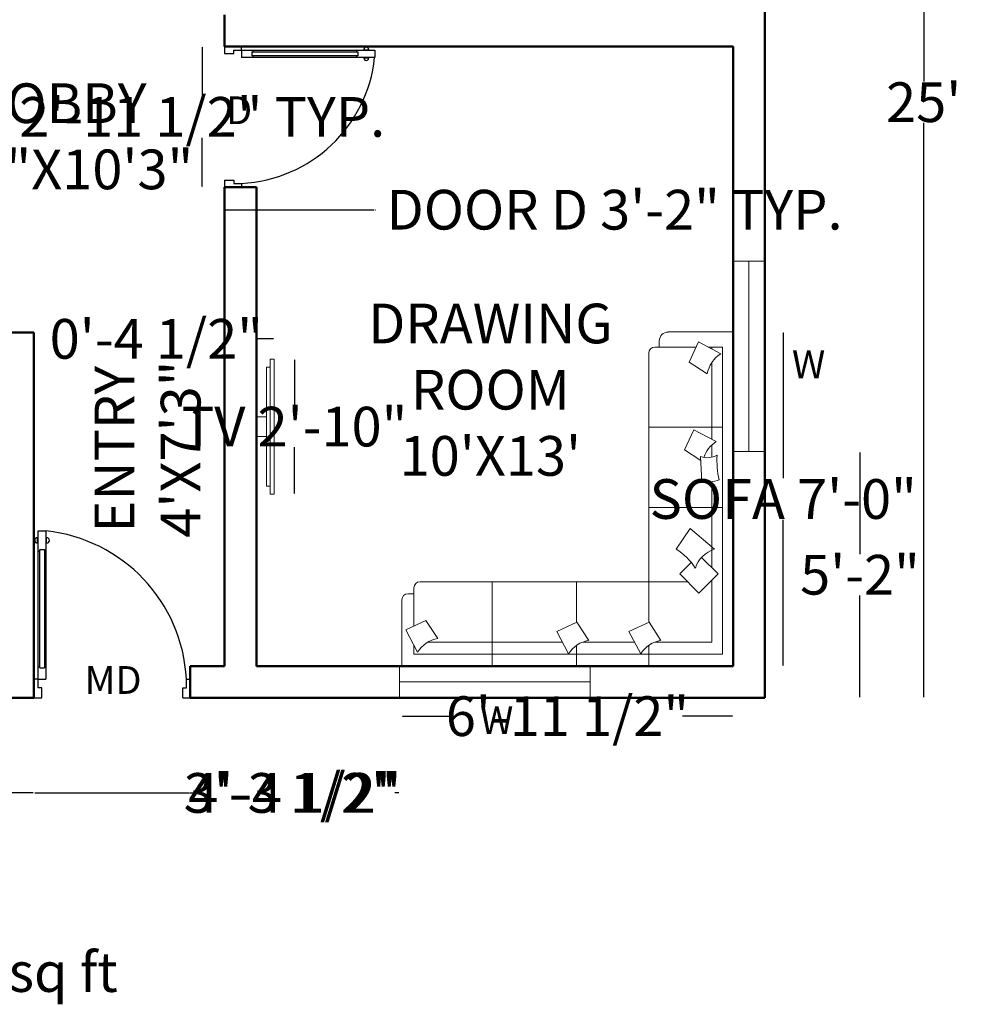
# Model space of a CAD drawing. Units: inches. Extents: x 387 to 883, y 95 to 571.
# Tile 2 of 3: x 646 to 883, y 95 to 343. Entities that reach past the tile are written whole.
import ezdxf

# ---------------------------------------------------------------- set-up
doc = ezdxf.new("R2010")
doc.units = ezdxf.units.IN
doc.header["$MEASUREMENT"] = 0
for name, color, linetype, lineweight in [('A-ANNO-DIMS', 2, 'Continuous', 18), ('A-ANNO-TEXT', 7, 'Continuous', 18), ('A-AREA-IDEN', 7, 'Continuous', 25), ('A-DOOR', 3, 'Continuous', 25), ('A-EQPM', 9, 'Continuous', 18), ('A-FURN', 8, 'Continuous', 18), ('A-GLAZ', 4, 'Continuous', 18), ('A-WALL', 7, 'Continuous', 50)]:
    doc.layers.add(name, color=color, linetype=linetype, lineweight=lineweight)
doc.styles.get("Standard").update_dxf_attribs({"font": 'arial.ttf'})
doc.dimstyles.get("Standard").update_dxf_attribs({"dimtxt": 10, "dimasz": 0.18, "dimexe": 0.18, "dimexo": 0.0625, "dimgap": 0.09, "dimtad": 0, "dimtih": 1, "dimtoh": 1, "dimdec": 0, "dimzin": 0, "dimdsep": 46, "dimlunit": 4, "dimtxsty": 'Standard', "dimcen": 0.09, "dimse1": 1, "dimse2": 1, "dimadec": 0, "dimazin": 0, "dimtfac": 1, "dimtdec": 0, "dimtofl": 0, "dimtmove": 0, "dimatfit": 3, "dimfxl": 1, "dimtolj": 1, "dimtzin": 0, "dimarcsym": 0})

# ---------------------------------------------------------------- blocks, each defined once
blk = doc.blocks.new('w')
blk.add_line((755.51, 424.04), (707.51, 424.04))
blk.add_lwpolyline([(707.51, 420.04), (755.51, 420.04), (755.51, 428.04), (707.51, 428.04)], close=True)
blk = doc.blocks.new('d1')
for p, q in [((2995.6, 698.54), (2995.6, 699.83)), ((2995.74, 701.33), (2997.52, 701.33)), ((2995.74, 667.71), (2995.74, 701.33)), ((2997.52, 701.33), (2997.52, 667.71)), ((2997.66, 698.54), (2997.66, 699.83)), ((2996.1, 697.09), (2997.16, 697.09)), ((2996.1, 670.28), (2996.1, 697.09)), ((2997.16, 697.09), (2997.16, 670.28)), ((2995.74, 696.72), (2996.1, 696.72)), ((2997.16, 696.72), (2997.52, 696.72)), ((2995.74, 670.55), (2996.1, 670.55)), ((2996.1, 670.28), (2997.16, 670.28)), ((2997.16, 670.55), (2997.52, 670.55)), ((2995.74, 667.71), (2994.8, 667.71)), ((2994.8, 663.45), (2994.8, 667.71)), ((2995.74, 667.71), (2997.52, 667.71)), ((2995.74, 665.76), (2995.74, 667.71)), ((3029.37, 665.76), (3029.37, 667.71)), ((3029.37, 667.71), (3030.3, 667.71)), ((3030.3, 663.45), (3030.3, 667.71)), ((2996.58, 665.76), (2995.74, 665.76)), ((2996.58, 663.45), (2996.58, 665.76)), ((3028.53, 665.76), (3029.37, 665.76)), ((3028.53, 663.45), (3028.53, 665.76)), ((2994.8, 663.45), (2996.58, 663.45)), ((3028.53, 663.45), (3030.3, 663.45))]:
    blk.add_line(p, q)
for centre, radius, start, end in [((2995.6, 699.19), 0.641, 90, 270), ((2993.79, 665.9), 35.62, 2.9057, 83.9884), ((2997.66, 699.19), 0.641, 270, 90)]:
    blk.add_arc(centre, radius, start, end)
blk = doc.blocks.new('sa')
at = {"color": 0, "linetype": 'ByBlock'}
for p, q in [((970.64, 101.74), (986.94, 101.74)), ((986.94, 101.74), (986.94, 17.6)), ((968.37, 97.95), (968.37, 99.46)), ((975.91, 94.16), (978.25, 99.24)), ((978.25, 99.24), (983.85, 96.25)), ((967.23, 97.95), (968.37, 97.95)), ((977.66, 97.95), (968.37, 97.95)), ((984.29, 97.95), (980.68, 97.95)), ((981.63, 97.95), (981.63, 97.44)), ((984.29, 20.63), (984.29, 97.95)), ((965.72, 28.58), (965.72, 96.43)), ((980.46, 91.17), (975.91, 94.16)), ((981.63, 94.1), (981.63, 74.68)), ((965.72, 77.73), (984.29, 77.73)), ((974.74, 72.03), (977.08, 77.11)), ((977.08, 77.11), (982.68, 74.13)), ((978.81, 69.36), (974.74, 72.03)), ((981.63, 73.33), (981.63, 70.22)), ((979.04, 63.97), (978.77, 70.35)), ((981.63, 64.06), (981.63, 42.35)), ((965.72, 57.52), (984.29, 57.52)), ((976.16, 52.26), (972.61, 47.06)), ((982.26, 47.06), (976.16, 52.26)), ((983.18, 40.81), (979.02, 44.97)), ((976.41, 43.69), (973.53, 40.81)), ((973.53, 40.81), (978.35, 35.98)), ((978.35, 35.98), (983.18, 40.81)), ((906.59, 27.66), (906.59, 37.31)), ((908.11, 38.82), (975.52, 38.82)), ((926.3, 17.6), (926.3, 38.82)), ((947.52, 28.58), (947.52, 38.82)), ((981.63, 39.27), (981.63, 23.66)), ((905.08, 35.79), (906.59, 35.79)), ((903.56, 17.6), (903.56, 34.27)), ((909.62, 29.06), (904.54, 26.72)), ((912.61, 24.51), (909.62, 29.06)), ((947.61, 28.62), (942.53, 26.28)), ((950.6, 24.08), (947.61, 28.62)), ((965.81, 28.62), (960.73, 26.28)), ((965.81, 28.62), (960.73, 26.28)), ((968.79, 24.08), (965.81, 28.62)), ((968.79, 24.08), (965.81, 28.62)), ((904.54, 26.72), (907.53, 21.12)), ((942.53, 26.28), (945.52, 20.69)), ((960.73, 26.28), (963.71, 20.69)), ((960.73, 26.28), (963.71, 20.69)), ((906.59, 20.63), (906.59, 22.88)), ((940.9, 23.66), (910.22, 23.66)), ((947.52, 17.6), (947.52, 22.8)), ((965.72, 17.6), (965.72, 22.8)), ((981.63, 23.66), (967.31, 23.66)), ((963.06, 20.63), (906.59, 20.63)), ((965.72, 17.6), (903.56, 17.6))]:
    blk.add_line(p, q, dxfattribs=at)
for p, q in [((947.52, 38.82), (947.52, 28.58)), ((940.9, 23.66), (925.56, 23.66)), ((943.93, 23.66), (928.59, 23.66)), ((947.52, 22.8), (947.52, 17.6)), ((962.13, 23.66), (949.12, 23.66)), ((965.72, 22.8), (965.72, 17.6)), ((965.72, 22.8), (965.72, 17.6)), ((944.49, 20.63), (926.3, 20.63)), ((947.52, 20.63), (929.33, 20.63)), ((984.29, 20.63), (947.52, 20.63)), ((944.49, 17.6), (926.3, 17.6)), ((947.52, 17.6), (929.33, 17.6)), ((986.94, 17.6), (947.52, 17.6))]:
    blk.add_line(p, q)
for centre, radius, start, end in [((970.64, 99.46), 2.27, 90, 180), ((967.23, 96.43), 1.52, 90, 180), ((987.88, 89.89), 7.54, 122.3301, 170.157), ((986.71, 67.76), 7.54, 122.3301, 161.5057), ((980.42, 75.11), 5.04, 250.8325, 299.9235), ((1002.47, 69.24), 19.59, 175.599, 194.0402), ((979.94, 75.27), 11.34, 265.4155, 288.0697), ((964.63, 34.26), 15.08, 31.9301, 58.0699), ((984.6, 39.9), 7.53, 108.0785, 161.9215), ((908.11, 37.31), 1.52, 90, 180), ((905.08, 34.27), 1.52, 90, 180), ((913.9, 17.09), 7.54, 99.843, 147.6699), ((951.89, 16.66), 7.54, 99.843, 147.6699), ((970.08, 16.66), 7.54, 99.843, 147.6699), ((970.08, 16.66), 7.54, 99.843, 147.6699)]:
    blk.add_arc(centre, radius, start, end, dxfattribs=at)
blk = doc.blocks.new('tv')
for points in [[(973.08, 134.58), (978.08, 134.58), (978.08, 137.08), (973.08, 137.08)], [(960.58, 133.58), (990.58, 133.58), (990.58, 134.58), (960.58, 134.58)], [(958.58, 132.58), (992.58, 132.58), (992.58, 133.58), (958.58, 133.58)]]:
    blk.add_lwpolyline(points, close=True)
blk = doc.blocks.new('*D12')
at = {"layer": 'A-ANNO-DIMS', "color": 0, "lineweight": -2, "transparency": 16777216}
for p, q in [((873.84, 471.82), (873.84, 327.19)), ((873.84, 172.18), (873.84, 316.8))]:
    blk.add_line(p, q, dxfattribs=at)
at = {"layer": 'A-ANNO-DIMS', "color": 0, "transparency": 16777216}
for points in [[(873.81, 471.82), (873.87, 471.82), (873.84, 472)], [(873.81, 172.18), (873.87, 172.18), (873.84, 172)]]:
    blk.add_solid(points, dxfattribs=at)
at = {"layer": 'Defpoints', "color": 0, "transparency": 16777216}
for p in [(833.85, 472), (833.85, 172), (873.84, 172)]:
    blk.add_point(p, dxfattribs=at)
at = {"layer": 'A-ANNO-DIMS', "color": 0, "transparency": 16777216, "insert": (873.84, 322), "char_height": 10, "attachment_point": 5}
blk.add_mtext("\\A1;25'", dxfattribs=at)
blk = doc.blocks.new('*D19')
at = {"layer": 'A-ANNO-DIMS', "color": 0, "lineweight": -2, "transparency": 16777216}
for p, q in [((698.03, 294.93), (735.45, 294.93)), ((735.63, 294.93), (735.81, 294.93))]:
    blk.add_line(p, q, dxfattribs=at)
at = {"layer": 'A-ANNO-DIMS', "color": 0, "transparency": 16777216}
for points in [[(698.03, 294.96), (698.03, 294.9), (697.85, 294.93)], [(735.45, 294.96), (735.45, 294.9), (735.63, 294.93)]]:
    blk.add_solid(points, dxfattribs=at)
at = {"layer": 'Defpoints', "color": 0, "transparency": 16777216}
for p in [(697.85, 300.6), (735.63, 300.6), (735.63, 294.93)]:
    blk.add_point(p, dxfattribs=at)
at = {"layer": 'A-ANNO-DIMS', "color": 0, "transparency": 16777216, "insert": (796.01, 294.93), "char_height": 10, "attachment_point": 5}
blk.add_mtext('\\A1;DOOR D 3\'-2" TYP.', dxfattribs=at)
blk = doc.blocks.new('*D20')
at = {"layer": 'A-ANNO-DIMS', "color": 0, "lineweight": -2, "transparency": 16777216}
for p, q in [((692.19, 335.82), (692.19, 323.56)), ((692.19, 300.78), (692.19, 313.04))]:
    blk.add_line(p, q, dxfattribs=at)
at = {"layer": 'A-ANNO-DIMS', "color": 0, "transparency": 16777216}
for points in [[(692.16, 335.82), (692.22, 335.82), (692.19, 336)], [(692.16, 300.78), (692.22, 300.78), (692.19, 300.6)]]:
    blk.add_solid(points, dxfattribs=at)
at = {"layer": 'Defpoints', "color": 0, "transparency": 16777216}
for p in [(697.85, 336), (692.19, 300.6), (697.85, 300.6)]:
    blk.add_point(p, dxfattribs=at)
at = {"layer": 'A-ANNO-DIMS', "color": 0, "transparency": 16777216, "insert": (692.19, 318.3), "char_height": 10, "attachment_point": 5}
blk.add_mtext('\\A1;2\'-11 1/2" TYP.', dxfattribs=at)
blk = doc.blocks.new('*D29')
at = {"layer": 'A-ANNO-DIMS', "color": 0, "lineweight": -2, "transparency": 16777216}
for p, q in [((838.47, 263.96), (838.47, 227.33)), ((838.47, 180.18), (838.47, 216.8))]:
    blk.add_line(p, q, dxfattribs=at)
at = {"layer": 'A-ANNO-DIMS', "color": 0, "transparency": 16777216}
for points in [[(838.44, 263.96), (838.5, 263.96), (838.47, 264.14)], [(838.44, 180.18), (838.5, 180.18), (838.47, 180)]]:
    blk.add_solid(points, dxfattribs=at)
at = {"layer": 'Defpoints', "color": 0, "transparency": 16777216}
for p in [(825.85, 264.14), (838.47, 264.14), (825.85, 180)]:
    blk.add_point(p, dxfattribs=at)
at = {"layer": 'A-ANNO-DIMS', "color": 0, "transparency": 16777216, "insert": (838.47, 222.07), "char_height": 10, "attachment_point": 5}
blk.add_mtext('\\A1;SOFA 7\'-0"', dxfattribs=at)
blk = doc.blocks.new('*D30')
at = {"layer": 'A-ANNO-DIMS', "color": 0, "lineweight": -2, "transparency": 16777216}
for p, q in [((742.65, 167.38), (755.22, 167.38)), ((825.67, 167.38), (813.1, 167.38))]:
    blk.add_line(p, q, dxfattribs=at)
at = {"layer": 'A-ANNO-DIMS', "color": 0, "transparency": 16777216}
for points in [[(742.65, 167.41), (742.65, 167.35), (742.47, 167.38)], [(825.67, 167.41), (825.67, 167.35), (825.85, 167.38)]]:
    blk.add_solid(points, dxfattribs=at)
at = {"layer": 'Defpoints', "color": 0, "transparency": 16777216}
for p in [(742.47, 180), (825.85, 180), (825.85, 167.38)]:
    blk.add_point(p, dxfattribs=at)
at = {"layer": 'A-ANNO-DIMS', "color": 0, "transparency": 16777216, "insert": (784.16, 167.38), "char_height": 10, "attachment_point": 5}
blk.add_mtext('\\A1;6\'-11 1/2"', dxfattribs=at)
blk = doc.blocks.new('*D31')
at = {"layer": 'A-ANNO-DIMS', "color": 0, "lineweight": -2, "transparency": 16777216}
for p, q in [((715.45, 257.12), (715.45, 245.49)), ((715.45, 223.48), (715.45, 235.1))]:
    blk.add_line(p, q, dxfattribs=at)
at = {"layer": 'A-ANNO-DIMS', "color": 0, "transparency": 16777216}
for points in [[(715.42, 257.12), (715.48, 257.12), (715.45, 257.3)], [(715.42, 223.48), (715.48, 223.48), (715.45, 223.3)]]:
    blk.add_solid(points, dxfattribs=at)
at = {"layer": 'Defpoints', "color": 0, "transparency": 16777216}
for p in [(710.35, 257.3), (715.45, 257.3), (710.35, 223.3)]:
    blk.add_point(p, dxfattribs=at)
at = {"layer": 'A-ANNO-DIMS', "color": 0, "transparency": 16777216, "insert": (715.45, 240.3), "char_height": 10, "attachment_point": 5}
blk.add_mtext('\\A1;TV 2\'-10"', dxfattribs=at)
blk = doc.blocks.new('*D32')
at = {"layer": 'A-ANNO-DIMS', "color": 0, "lineweight": -2, "transparency": 16777216}
for p, q in [((705.85, 262.4), (705.67, 262.4)), ((710.17, 262.4), (706.03, 262.4))]:
    blk.add_line(p, q, dxfattribs=at)
at = {"layer": 'A-ANNO-DIMS', "color": 0, "transparency": 16777216}
for points in [[(706.03, 262.43), (706.03, 262.37), (705.85, 262.4)], [(710.17, 262.43), (710.17, 262.37), (710.35, 262.4)]]:
    blk.add_solid(points, dxfattribs=at)
at = {"layer": 'Defpoints', "color": 0, "transparency": 16777216}
for p in [(705.85, 262.4), (705.85, 257.3), (710.35, 257.3)]:
    blk.add_point(p, dxfattribs=at)
at = {"layer": 'A-ANNO-DIMS', "color": 0, "transparency": 16777216, "insert": (680.64, 262.4), "char_height": 10, "attachment_point": 5}
blk.add_mtext('\\A1;0\'-4 1/2"', dxfattribs=at)
blk = doc.blocks.new('*D37')
at = {"layer": 'A-ANNO-DIMS', "color": 0, "lineweight": -2, "transparency": 16777216}
for p, q in [((857.8, 233.82), (857.8, 208.19)), ((857.8, 172.18), (857.8, 197.8))]:
    blk.add_line(p, q, dxfattribs=at)
at = {"layer": 'A-ANNO-DIMS', "color": 0, "transparency": 16777216}
for points in [[(857.77, 233.82), (857.83, 233.82), (857.8, 234)], [(857.77, 172.18), (857.83, 172.18), (857.8, 172)]]:
    blk.add_solid(points, dxfattribs=at)
at = {"layer": 'Defpoints', "color": 0, "transparency": 16777216}
for p in [(833.85, 234), (857.8, 234), (833.85, 172)]:
    blk.add_point(p, dxfattribs=at)
at = {"layer": 'A-ANNO-DIMS', "color": 0, "transparency": 16777216, "insert": (857.8, 203), "char_height": 10, "attachment_point": 5}
blk.add_mtext('\\A1;5\'-2"', dxfattribs=at)
blk = doc.blocks.new('*D38')
at = {"layer": 'A-ANNO-DIMS', "color": 0, "lineweight": -2, "transparency": 16777216}
for p, q in [((462.03, 148.05), (539.06, 148.05)), ((649.67, 148.05), (572.65, 148.05))]:
    blk.add_line(p, q, dxfattribs=at)
at = {"layer": 'A-ANNO-DIMS', "color": 0, "transparency": 16777216}
for points in [[(462.03, 148.08), (462.03, 148.02), (461.85, 148.05)], [(649.67, 148.08), (649.67, 148.02), (649.85, 148.05)]]:
    blk.add_solid(points, dxfattribs=at)
at = {"layer": 'Defpoints', "color": 0, "transparency": 16777216}
for p in [(461.85, 172), (649.85, 172), (649.85, 148.05)]:
    blk.add_point(p, dxfattribs=at)
at = {"layer": 'A-ANNO-DIMS', "color": 0, "transparency": 16777216, "insert": (555.85, 148.05), "char_height": 10, "attachment_point": 5}
blk.add_mtext('\\A1;15\'-8"', dxfattribs=at)
blk = doc.blocks.new('*D39')
at = {"layer": 'A-ANNO-DIMS', "color": 0, "lineweight": -2, "transparency": 16777216}
for p, q in [((689.33, 148.05), (690.27, 148.05)), ((741.67, 148.05), (740.73, 148.05))]:
    blk.add_line(p, q, dxfattribs=at)
at = {"layer": 'A-ANNO-DIMS', "color": 0, "transparency": 16777216}
for points in [[(689.33, 148.08), (689.33, 148.02), (689.15, 148.05)], [(741.67, 148.08), (741.67, 148.02), (741.85, 148.05)]]:
    blk.add_solid(points, dxfattribs=at)
at = {"layer": 'Defpoints', "color": 0, "transparency": 16777216}
for p in [(689.15, 172), (741.85, 172), (741.85, 148.05)]:
    blk.add_point(p, dxfattribs=at)
at = {"layer": 'A-ANNO-DIMS', "color": 0, "transparency": 16777216, "insert": (715.5, 148.05), "char_height": 10, "attachment_point": 5}
blk.add_mtext('\\A1;4\'-4 1/2"', dxfattribs=at)
blk = doc.blocks.new('*D42')
at = {"layer": 'A-ANNO-DIMS', "color": 0, "lineweight": -2, "transparency": 16777216}
for p, q in [((650.03, 148.05), (688.97, 148.05)), ((689.15, 148.05), (689.33, 148.05))]:
    blk.add_line(p, q, dxfattribs=at)
at = {"layer": 'A-ANNO-DIMS', "color": 0, "transparency": 16777216}
for points in [[(650.03, 148.08), (650.03, 148.02), (649.85, 148.05)], [(688.97, 148.08), (688.97, 148.02), (689.15, 148.05)]]:
    blk.add_solid(points, dxfattribs=at)
at = {"layer": 'Defpoints', "color": 0, "transparency": 16777216}
for p in [(649.85, 172), (689.15, 172), (689.15, 148.05)]:
    blk.add_point(p, dxfattribs=at)
at = {"layer": 'A-ANNO-DIMS', "color": 0, "transparency": 16777216, "insert": (714.36, 148.05), "char_height": 10, "attachment_point": 5}
blk.add_mtext('\\A1;3\'-3 1/2"', dxfattribs=at)
blk = doc.blocks.new('*D43')
at = {"layer": 'A-ANNO-DIMS', "color": 0, "lineweight": -2, "transparency": 16777216}
for p, q in [((437.9, 213.86), (437.9, 198.22)), ((437.9, 172.18), (437.9, 187.82))]:
    blk.add_line(p, q, dxfattribs=at)
at = {"layer": 'A-ANNO-DIMS', "color": 0, "transparency": 16777216}
for points in [[(437.87, 213.86), (437.93, 213.86), (437.9, 214.04)], [(437.87, 172.18), (437.93, 172.18), (437.9, 172)]]:
    blk.add_solid(points, dxfattribs=at)
at = {"layer": 'Defpoints', "color": 0, "transparency": 16777216}
for p in [(437.9, 214.04), (650.89, 214.04), (649.85, 172)]:
    blk.add_point(p, dxfattribs=at)
at = {"layer": 'A-ANNO-DIMS', "color": 0, "transparency": 16777216, "insert": (437.9, 193.02), "char_height": 10, "attachment_point": 5}
blk.add_mtext('\\A1;3\'-6"', dxfattribs=at)

msp = doc.modelspace()

# ---------------------------------------------------------------- linework, layer by layer
at = {"layer": 'A-WALL'}
for p, q in [((833.85, 172), (833.85, 472)), ((697.85, 336), (697.85, 344)), ((697.85, 336), (825.85, 336)), ((825.85, 180), (825.85, 336)), ((697.85, 180), (697.85, 300.6)), ((697.85, 300.6), (705.85, 300.6)), ((705.85, 180), (705.85, 300.6)), ((589.85, 264), (649.85, 264)), ((649.85, 172), (649.85, 264)), ((689.15, 180), (697.85, 180)), ((689.15, 172), (689.15, 180)), ((705.85, 180), (825.85, 180)), ((461.85, 172), (649.85, 172)), ((689.15, 172), (833.85, 172))]:
    msp.add_line(p, q, dxfattribs=at)

# ---------------------------------------------------------------- block references
at = {"layer": 'A-DOOR', "xscale": 0.9971830985915492, "yscale": 0.9971830985915492, "zscale": 0.9971830985915492, "rotation": 270}
msp.add_blockref('d1', (36.27, 3322.37), dxfattribs=at)
at = {"layer": 'A-DOOR', "xscale": 1.109859154929577, "yscale": 1.109859154929577, "zscale": 1.109859154929577}
msp.add_blockref('d1', (-2673.96, -564.34), dxfattribs=at)
at = {"layer": 'A-EQPM', "rotation": 90}
msp.add_blockref('tv', (842.93, -735.28), dxfattribs=at)
at = {"layer": 'A-FURN'}
msp.add_blockref('sa', (-161.09, 162.4), dxfattribs=at)
at = {"layer": 'A-GLAZ', "rotation": 90}
msp.add_blockref('w', (1253.89, -473.51), dxfattribs=at)
at = {"layer": 'A-GLAZ'}
msp.add_blockref('w', (34.34, -248.04), dxfattribs=at)

# ---------------------------------------------------------------- texts
at = {"layer": 'A-ANNO-TEXT', "attachment_point": 1}
for s, width, insert, char_height in [('\\pxqc;D', 47.8337, (677.58, 323.47), 7), ('\\pxqc;W', 47.8337, (820.95, 259.5), 7), ('\\pxqc;MD', 47.8337, (645.85, 180), 7), ('\\pxqc;W', 47.8337, (742.43, 169.89), 7), ('TOTAL BUILD UP AREA-775 sq ft', 214.2919, (470.27, 107.95), 10)]:
    msp.add_mtext_dynamic_manual_height_columns(s, width=width, gutter_width=1, heights=[0], dxfattribs=dict(at, insert=insert, char_height=char_height))
at = {"layer": 'A-AREA-IDEN', "char_height": 10, "attachment_point": 1}
for s, insert in [('\\pxqc;LOBBY\\P8\'6"X10\'3"', (632.93, 326.75)), ("\\pxqc;DRAWING ROOM\\P10'X13'", (740.83, 271.27))]:
    msp.add_mtext_dynamic_manual_height_columns(s, width=47.8337, gutter_width=1, heights=[0], dxfattribs=dict(at, insert=insert))
at = {"layer": 'A-AREA-IDEN', "insert": (665.1, 210.71), "char_height": 10, "attachment_point": 1, "rotation": 90}
msp.add_mtext_dynamic_manual_height_columns('\\pxqc;ENTRY\\P4\'X7\'3"', width=47.8337, gutter_width=1, heights=[0], dxfattribs=at)

# ---------------------------------------------------------------- dimensions: what is measured, and where the dimension line sits
at = {"layer": 'A-ANNO-DIMS'}
dim = msp.add_aligned_dim(p1=(833.85, 472), p2=(833.85, 172), distance=39.99, dimstyle='Standard', override={"dimclrd": 0, "dimclre": 0, "dimclrt": 0}, dxfattribs=at)
dim.commit()
dim.dimension.update_dxf_attribs({"geometry": '*D12', "text_midpoint": (873.84, 322)})
for base, p1, p2, angle, text, picture, middle in [((692.19, 300.6), (697.85, 336), (697.85, 300.6), 270, '<> TYP.', '*D20', (692.19, 318.3)), ((838.47, 264.14), (825.85, 180), (825.85, 264.14), 90, 'SOFA <>', '*D29', (838.47, 222.07)), ((715.45, 257.3), (710.35, 223.3), (710.35, 257.3), 90, 'TV <>', '*D31', (715.45, 240.3))]:
    dim = msp.add_linear_dim(base=base, p1=p1, p2=p2, angle=angle, text=text, dimstyle='Standard', override={"dimdec": 1, "dimlfac": 1, "dimrnd": 0, "dimzin": 1, "dimdsep": 46, "dimlunit": 4, "dimfrac": 2}, dxfattribs=at)
    dim.commit()
    dim.dimension.update_dxf_attribs({"geometry": picture, "text_midpoint": middle})
dim = msp.add_linear_dim(base=(735.63, 294.93), p1=(697.85, 300.6), p2=(735.63, 300.6), text='DOOR D <> TYP.', dimstyle='Standard', override={"dimdec": 1, "dimlfac": 1, "dimrnd": 0, "dimzin": 1, "dimdsep": 46, "dimlunit": 4, "dimfrac": 2}, dxfattribs=at)
dim.commit()
dim.dimension.update_dxf_attribs({"geometry": '*D19', "text_midpoint": (796.01, 294.93)})
for base, p1, p2, angle, picture, middle in [((705.85, 262.4), (710.35, 257.3), (705.85, 257.3), 180, '*D32', (680.64, 262.4)), ((857.8, 234), (833.85, 172), (833.85, 234), 90, '*D37', (857.8, 203)), ((437.9, 214.04), (649.85, 172), (650.89, 214.04), 90, '*D43', (437.9, 193.02))]:
    dim = msp.add_linear_dim(base=base, p1=p1, p2=p2, angle=angle, dimstyle='Standard', override={"dimdec": 1, "dimlfac": 1, "dimrnd": 0, "dimzin": 1, "dimdsep": 46, "dimlunit": 4, "dimfrac": 2}, dxfattribs=at)
    dim.commit()
    dim.dimension.update_dxf_attribs({"geometry": picture, "text_midpoint": middle})
for base, p1, p2, picture, middle in [((825.85, 167.38), (742.47, 180), (825.85, 180), '*D30', (784.16, 167.38)), ((649.85, 148.05), (461.85, 172), (649.85, 172), '*D38', (555.85, 148.05)), ((689.15, 148.05), (649.85, 172), (689.15, 172), '*D42', (714.36, 148.05)), ((741.85, 148.05), (689.15, 172), (741.85, 172), '*D39', (715.5, 148.05))]:
    dim = msp.add_linear_dim(base=base, p1=p1, p2=p2, dimstyle='Standard', override={"dimdec": 1, "dimlfac": 1, "dimrnd": 0, "dimzin": 1, "dimdsep": 46, "dimlunit": 4, "dimfrac": 2}, dxfattribs=at)
    dim.commit()
    dim.dimension.update_dxf_attribs({"geometry": picture, "text_midpoint": middle})

doc.saveas('drawing.dxf')
